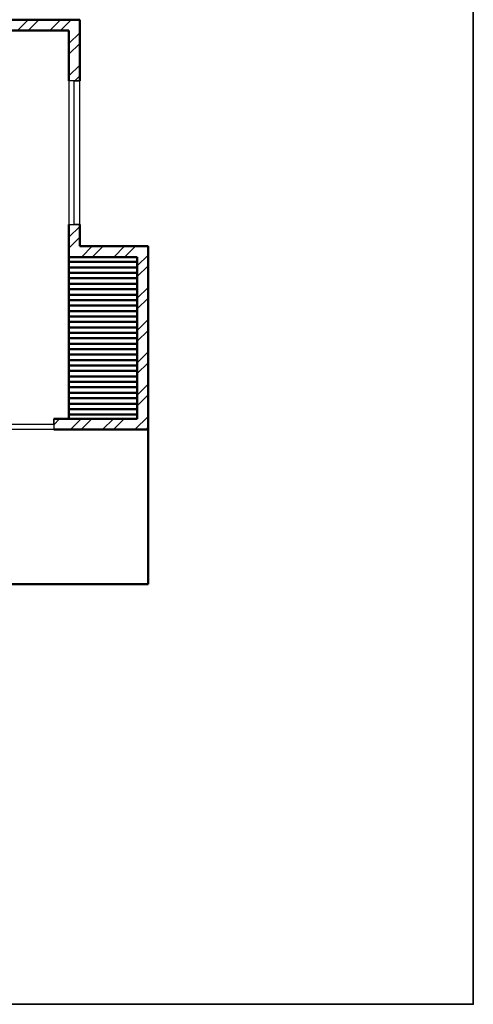
# Model space of a CAD drawing. Units: inches. Extents: x 963 to 2075, y 289 to 2657.
# Tile 47 of 98: x 1885 to 2075, y 1303 to 1714. Entities that reach past the tile are written whole.
import ezdxf

# ---------------------------------------------------------------- set-up
doc = ezdxf.new("R2010")
doc.units = ezdxf.units.IN
for name, color, linetype, lineweight in [('A-ANNO-TTLB', 7, 'Continuous', 35), ('A-GLAZ', 3, 'Continuous', 25), ('A-WALL', 7, 'Continuous', 50), ('A-WALL-PATT', 8, 'Continuous', 13)]:
    doc.layers.add(name, color=color, linetype=linetype, lineweight=lineweight)

msp = doc.modelspace()

# ---------------------------------------------------------------- hatches: boundary and pattern name
at = {"layer": 'A-WALL-PATT'}
h = msp.add_hatch(dxfattribs=at)
h.set_pattern_fill('ANSI32', color=256)
h.paths.add_polyline_path([(1910.42, 1929.42), (1910.42, 1963.51), (1905.92, 1963.51), (1905.92, 1929.42), (1845.92, 1929.42), (1845.92, 1993.37), (1843.67, 1993.37), (1841.42, 1993.37), (1841.42, 1951.16), (1841.42, 1924.92), (1853.42, 1924.92), (1853.42, 1913.07), (1857.92, 1913.07), (1857.92, 1924.92), (1910.42, 1924.92)])
h.paths.add_polyline_path([(1857.92, 1853.07), (1853.42, 1853.07), (1853.42, 1826.32), (1841.42, 1826.32), (1674.48, 1826.32), (1674.48, 1821.82), (1853.42, 1821.82), (1857.92, 1821.82)])
h.paths.add_polyline_path([(1857.92, 1821.82), (1853.42, 1821.82), (1853.42, 1807.79), (1857.92, 1807.79)])
h.paths.add_polyline_path([(1857.92, 1747.79), (1853.42, 1747.79), (1853.42, 1713.82), (1809.34, 1713.82), (1809.34, 1709.32), (1905.92, 1709.32), (1905.92, 1688.32), (1910.42, 1688.32), (1910.42, 1713.82), (1857.92, 1713.82)])
h.paths.add_polyline_path([(1830.92, 1542.82), (1837.43, 1542.82), (1837.43, 1545.07), (1837.43, 1547.32), (1823.42, 1547.32), (1823.42, 1545.07), (1823.42, 1542.82), (1826.42, 1542.82), (1826.42, 1482.82), (1742.42, 1482.82), (1742.42, 1505.39), (1737.92, 1505.39), (1737.92, 1478.32), (1830.92, 1478.32)])
h.paths.add_polyline_path([(1938.92, 1619.32), (1934.42, 1619.32), (1910.42, 1619.32), (1910.42, 1628.32), (1908.17, 1628.32), (1905.92, 1628.32), (1905.92, 1614.82), (1934.42, 1614.82), (1934.42, 1547.32), (1905.92, 1547.32), (1899.59, 1547.32), (1899.59, 1542.82), (1910.42, 1542.82), (1938.92, 1542.82)])
h.paths.add_polyline_path([(1803.68, 1547.32), (1773.92, 1547.32), (1773.92, 1709.32), (1777.76, 1709.32), (1777.76, 1713.82), (1701.92, 1713.82), (1701.92, 1697.8), (1706.42, 1697.8), (1706.42, 1709.32), (1769.42, 1709.32), (1769.42, 1662.82), (1706.42, 1662.82), (1706.42, 1674.38), (1701.92, 1674.38), (1701.92, 1662.82), (1675.67, 1662.82), (1675.67, 1658.32), (1769.42, 1658.32), (1769.42, 1547.32), (1729.17, 1547.32), (1729.17, 1542.82), (1737.92, 1542.82), (1737.92, 1529.39), (1742.42, 1529.39), (1742.42, 1542.82), (1803.68, 1542.82)])
h.paths.add_polyline_path([(1595.42, 1542.82), (1599.24, 1542.82), (1599.24, 1547.32), (1584.36, 1547.32), (1584.36, 1542.82), (1590.92, 1542.82), (1590.92, 1436.32), (1595.42, 1436.32), (1595.42, 1440.82)])
h.paths.add_polyline_path([(1693.17, 1547.32), (1649.42, 1547.32), (1649.42, 1658.32), (1652.1, 1658.32), (1652.1, 1660.57), (1652.1, 1662.82), (1649.42, 1662.82), (1649.42, 1680.94), (1647.17, 1680.94), (1644.92, 1680.94), (1644.92, 1547.32), (1622.42, 1547.32), (1622.42, 1545.07), (1622.42, 1542.82), (1649.42, 1542.82), (1679.42, 1542.82), (1679.42, 1529.85), (1681.67, 1529.85), (1683.92, 1529.85), (1683.92, 1542.82), (1693.17, 1542.82), (1693.17, 1545.07)])
h.paths.add_polyline_path([(1683.92, 1505.85), (1679.42, 1505.85), (1679.42, 1483.8), (1595.42, 1483.8), (1595.42, 1479.3), (1683.92, 1479.3)])
h.paths.add_polyline_path([(1402.99, 1547.32), (1376.42, 1547.32), (1376.42, 1675.89), (1374.17, 1675.89), (1371.92, 1675.89), (1371.92, 1662.82), (1368.88, 1662.82), (1368.88, 1658.32), (1371.92, 1658.32), (1371.92, 1547.32), (1335.46, 1547.32), (1335.46, 1542.82), (1337.42, 1542.82), (1337.42, 1526.73), (1341.92, 1526.73), (1341.92, 1542.82), (1371.92, 1542.82), (1402.99, 1542.82)])

# ---------------------------------------------------------------- linework, layer by layer
at = {"layer": 'A-ANNO-TTLB'}
msp.add_lwpolyline([(962.81, 2657.49), (2074.6, 2657.49), (2074.6, 1303.08), (962.81, 1303.08)], close=True, dxfattribs=at)
at = {"layer": 'A-GLAZ'}
for p, q in [((1910.42, 1688.32), (1905.92, 1688.32)), ((1905.92, 1688.32), (1905.92, 1628.32)), ((1908.17, 1628.32), (1908.17, 1688.32)), ((1908.17, 1688.32), (1910.42, 1688.32)), ((1910.42, 1628.32), (1910.42, 1688.32)), ((1905.92, 1628.32), (1910.42, 1628.32)), ((1910.42, 1628.32), (1908.17, 1628.32)), ((1837.43, 1545.07), (1899.59, 1545.07)), ((1899.59, 1545.07), (1899.59, 1547.32)), ((1899.59, 1547.32), (1899.59, 1542.82)), ((1899.59, 1542.82), (1855.9, 1542.82))]:
    msp.add_line(p, q, dxfattribs=at)
at = {"layer": 'A-WALL'}
for p, q in [((1857.92, 1713.82), (1910.42, 1713.82)), ((1910.42, 1713.82), (1910.42, 1688.32)), ((1905.92, 1709.32), (1807.85, 1709.32)), ((1905.92, 1709.32), (1905.92, 1688.32)), ((1905.92, 1628.32), (1905.92, 1547.32)), ((1910.42, 1628.32), (1910.42, 1619.32)), ((1910.42, 1619.32), (1934.42, 1619.32)), ((1934.42, 1619.32), (1938.92, 1619.32)), ((1938.92, 1619.32), (1938.92, 1542.82)), ((1934.42, 1614.82), (1905.92, 1614.82)), ((1934.42, 1547.32), (1934.42, 1614.82)), ((1934.42, 1612.75), (1905.92, 1612.75)), ((1934.42, 1610.48), (1905.92, 1610.48)), ((1934.42, 1608.21), (1905.92, 1608.21)), ((1934.42, 1605.93), (1905.92, 1605.93)), ((1934.42, 1603.66), (1905.92, 1603.66)), ((1934.42, 1601.39), (1905.92, 1601.39)), ((1934.42, 1599.11), (1905.92, 1599.11)), ((1934.42, 1596.84), (1905.92, 1596.84)), ((1934.42, 1594.57), (1905.92, 1594.57)), ((1934.42, 1592.29), (1905.92, 1592.29)), ((1934.42, 1590.02), (1905.92, 1590.02)), ((1934.42, 1587.75), (1905.92, 1587.75)), ((1934.42, 1585.47), (1905.92, 1585.47)), ((1934.42, 1583.2), (1905.92, 1583.2)), ((1934.42, 1580.93), (1905.92, 1580.93)), ((1934.42, 1578.65), (1905.92, 1578.65)), ((1934.42, 1576.38), (1905.92, 1576.38)), ((1934.42, 1574.11), (1905.92, 1574.11)), ((1934.42, 1571.83), (1905.92, 1571.83)), ((1934.42, 1569.56), (1905.92, 1569.56)), ((1934.42, 1567.28), (1905.92, 1567.28)), ((1934.42, 1565.01), (1905.92, 1565.01)), ((1934.42, 1562.74), (1905.92, 1562.74)), ((1934.42, 1560.46), (1905.92, 1560.46)), ((1934.42, 1558.19), (1905.92, 1558.19)), ((1934.42, 1555.92), (1905.92, 1555.92)), ((1934.42, 1553.64), (1905.92, 1553.64)), ((1934.42, 1551.37), (1905.92, 1551.37)), ((1934.42, 1549.1), (1905.92, 1549.1)), ((1905.92, 1547.32), (1899.59, 1547.32)), ((1905.92, 1547.32), (1934.42, 1547.32)), ((1910.42, 1542.82), (1899.59, 1542.82)), ((1910.42, 1542.82), (1938.92, 1542.82)), ((1938.92, 1542.82), (1938.92, 1482.82)), ((1938.92, 1478.32), (1938.92, 1482.82)), ((1737.92, 1478.32), (1938.92, 1478.32)), ((1938.92, 1478.32), (1934.42, 1478.32))]:
    msp.add_line(p, q, dxfattribs=at)

doc.saveas('drawing.dxf')
